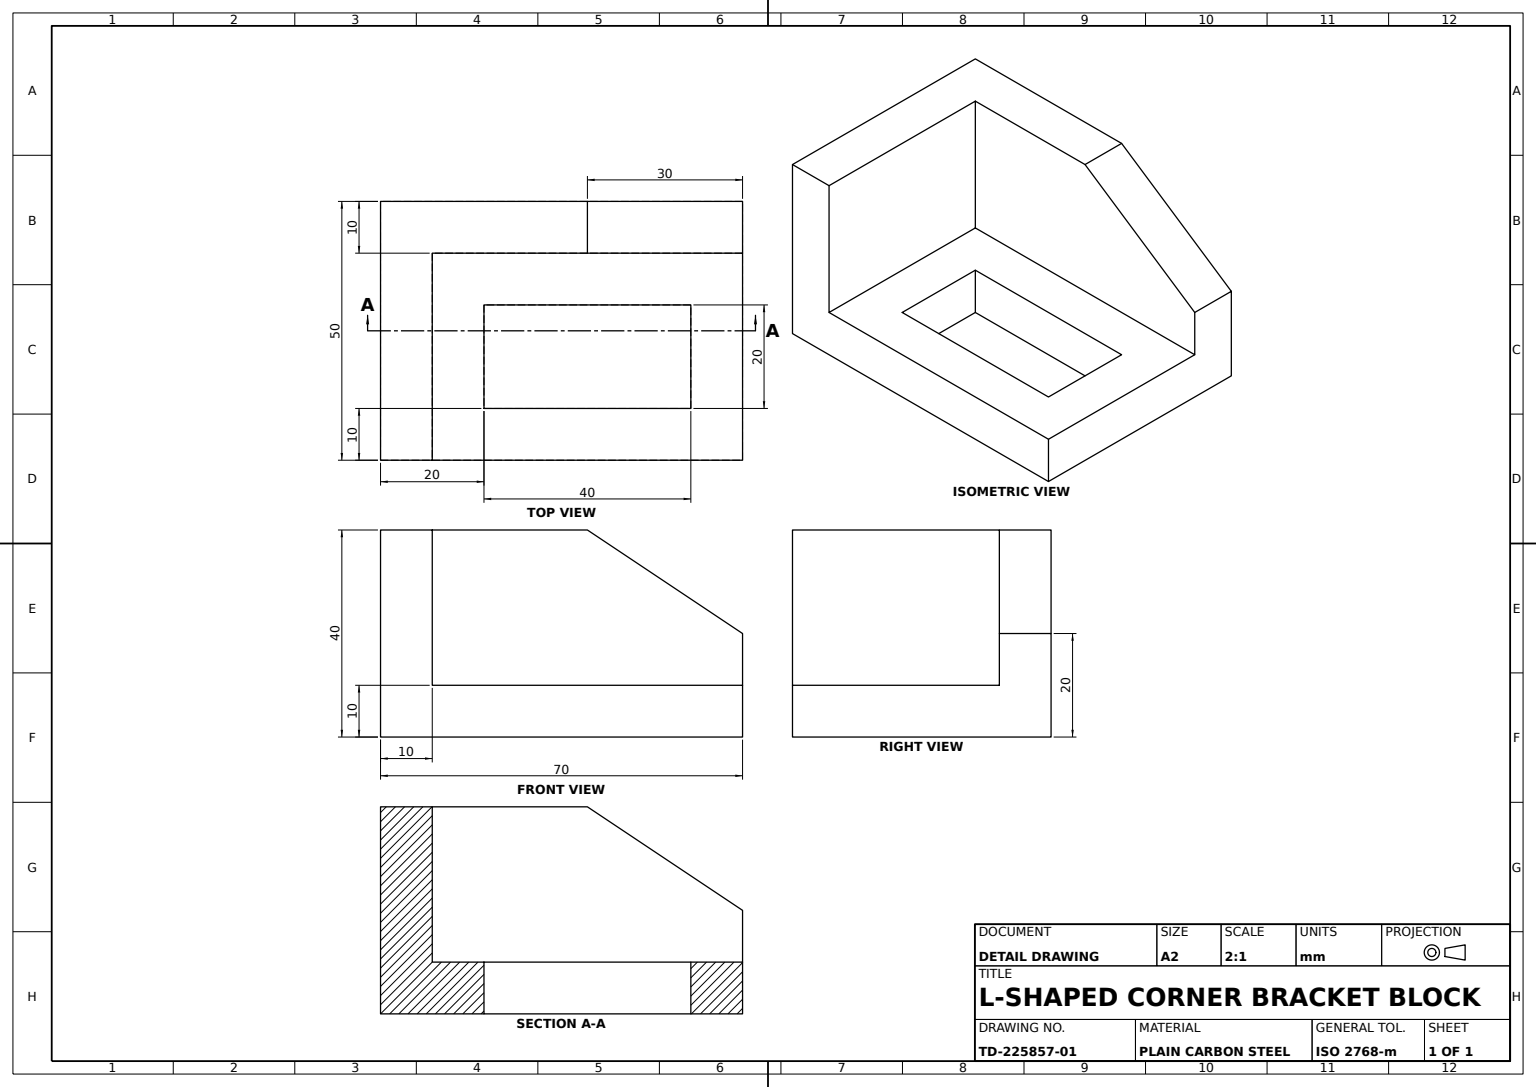
SolidWorks part; units mm, degrees
material "Plain Carbon Steel"
ref_plane "Front Plane" through (0, 0, 0) normal (0, 0, 1) x (1, 0, 0)
ref_plane "Top Plane" through (0, 0, 0) normal (0, 1, 0) x (1, 0, 0)
ref_plane "Right Plane" through (0, 0, 0) normal (1, 0, 0) x (0, 0, -1)
sketch "End Wall Profile Sketch" plane through (0, 0, 0) normal (0, 0, 1) x (1, 0, 0)
  line L0 (0, 0) -> (0, 40)
  line L1 (0, 40) -> (40, 40)
  line L2 (0, 0) -> (70, 0)
  line L3 (70, 0) -> (70, 20)
  line L4 (70, 20) -> (40, 40)
  dimension "D1" = 20
  dimension "D2" = 70
  dimension "D3" = 30
  dimension "D5" = 20
extrude "Chamfered End Wall" add sketch "End Wall Profile Sketch" along normal blind 10
sketch "Back Wall Sketch" plane through (0, 0, 10) normal (0, 0, 1) x (1, 0, 0)
  line L0 (0, 0) -> (70, 0) construction
  line L1 (0, 40) -> (10, 40)
  line L2 (0, 40) -> (0, 0)
  line L3 (0, 0) -> (10, 0)
  line L4 (10, 40) -> (10, 0)
  dimension "D1" = 10
extrude "Back Wall" add sketch "Back Wall Sketch" along normal blind 40
sketch "Base Plate Sketch" plane through (0, 0, 10) normal (0, 0, 1) x (1, 0, 0)
  line L0 (70, 0) -> (70, 20) construction
  line L1 (10, 0) -> (70, 0)
  line L2 (10, 0) -> (10, 10)
  line L3 (10, 10) -> (70, 10)
  line L4 (70, 0) -> (70, 10)
  dimension "D1" = 10
extrude "Base Plate" add sketch "Base Plate Sketch" along normal blind 40
sketch "Base Slot Sketch" plane through (0, 10, 0) normal (0, 1, 0) x (1, 0, 0)
  line L0 (70, -10) -> (10, -10) construction
  line L1 (20, -20) -> (60, -20)
  line L2 (20, -20) -> (20, -40)
  line L3 (20, -40) -> (60, -40)
  line L4 (60, -20) -> (60, -40)
  line L5 (70, -50) -> (70, -10) construction
  point P8 (70, -30)
  dimension "D1" = 40
  dimension "D2" = 20
  dimension "D3" = 10
  dimension "D4" = 10
extrude "Base Slot 40x20" cut sketch "Base Slot Sketch" against normal blind 10
